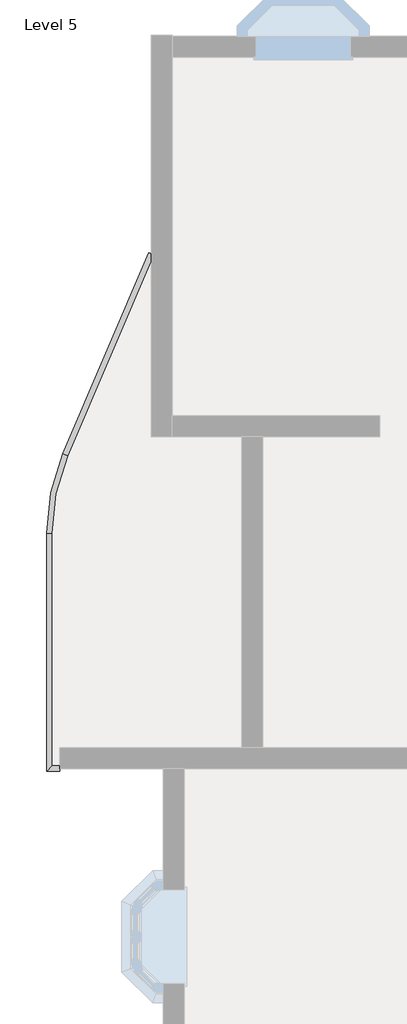
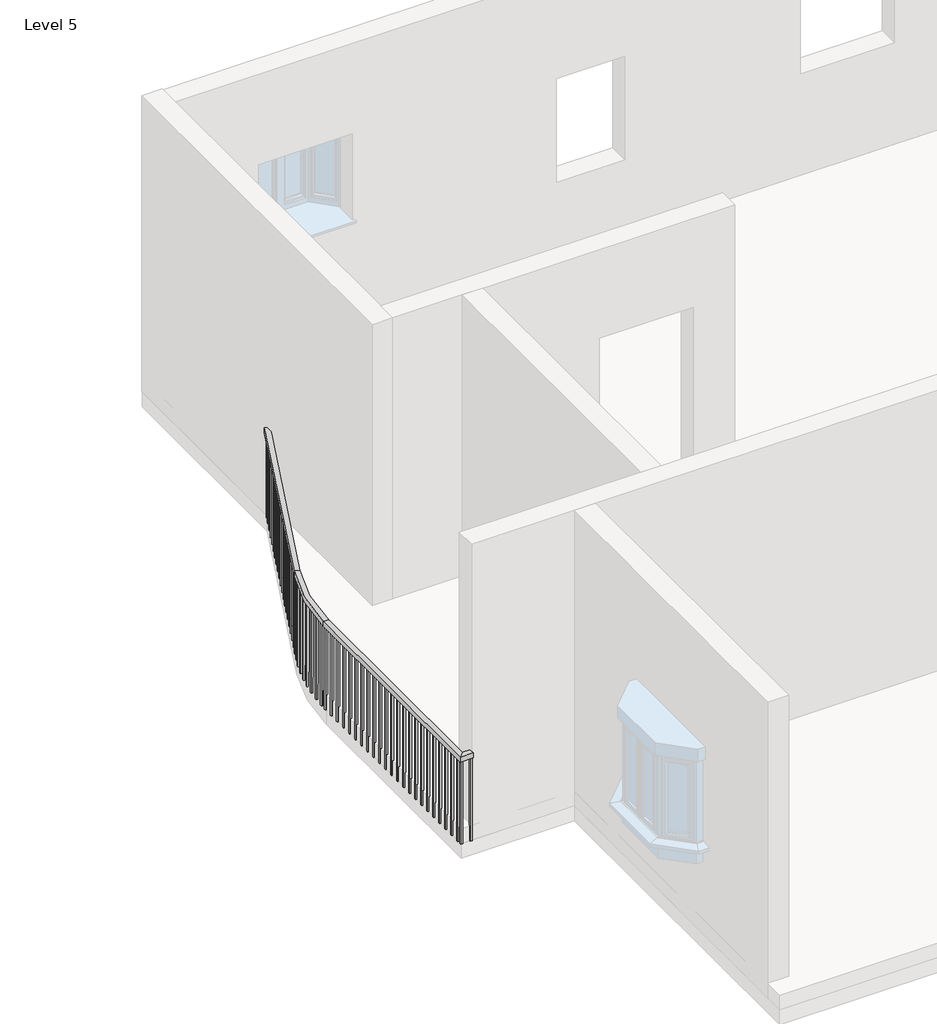
# One storey, part 7 of 14: 1 railing.
"""IFC4 building model written with IfcOpenShell, lengths in millimetres."""

from ifc_helpers import new_model, si_unit, frame, origin, place, context, project, spatial, polyline, circle_curve, outline, extrude, element, save
from ifc_brep_helpers import plane_surface, cylinder_surface, revolved_surface, advanced_brep

model = new_model("IFC4")

# Units and contexts
model_context = context("Model", 3, world=origin())
ifc_project = project(units=[si_unit("LENGTHUNIT", "METRE", prefix="MILLI")], contexts=[model_context])

# Site, building, storey
site = spatial("IfcSite", under=ifc_project)
building = spatial("IfcBuilding", under=site)
storey = spatial("IfcBuildingStorey", under=building, Name="Level 5", Elevation=12192.0)

# Railing
placement = place(None, origin())
element("IfcRailing", 1, ObjectType="Handrail - Rectangular", at=placement, inside=storey, context=model_context, shape_type="SolidModel", body=[
    advanced_brep(
    [(-12381.4379579, -2441.2590879, 13106.4), (-12381.4379579, -2441.2590879, 13055.6), (-12428.1364721, -2421.2618688, 13055.6), (-12428.1364721, -2421.2618688, 13106.4), (-13216.1814979, -4390.5942894, 13106.4), (-13216.1814979, -4390.5942894, 13055.6), (-13262.8800121, -4370.5970703, 13055.6), (-13262.8800121, -4370.5970703, 13106.4), (-13369.987215, -5140.4900045, 13055.6), (-13369.987215, -5140.4900045, 13106.4), (-13420.787215, -5140.4900045, 13055.6), (-13420.787215, -5140.4900045, 13106.4), (-13369.987215, -7396.5416506, 13106.4), (-13369.987215, -7396.5416506, 13055.6), (-13420.787215, -7447.3416506, 13055.6), (-13420.787215, -7447.3416506, 13106.4), (-13293.787215, -7396.5416506, 13106.4), (-13293.787215, -7447.3416506, 13106.4), (-13293.787215, -7447.3416506, 13055.6), (-13293.787215, -7396.5416506, 13055.6)],
    [
        (0, 1),
        (1, 2),
        (2, 3),
        (3, 0),
        (0, 4),
        (4, 5),
        (5, 1),
        (5, 6),
        (6, 2),
        (6, 7),
        (7, 3),
        (7, 4),
        (8, 5, circle_curve(frame((-11464.987215, -5140.4900045, 13055.6), z_axis=(0.0, 0.0, -1.0), x_axis=(-0.9192620907623801, 0.39364604467361003, 0.0)), 1905.0)),
        (4, 9, circle_curve(frame((-11464.987215, -5140.4900045, 13106.4), z_axis=(0.0, 0.0, 1.0), x_axis=(-0.9192620907623801, 0.39364604467361003, 0.0)), 1905.0)),
        (9, 8),
        (10, 6, circle_curve(frame((-11464.987215, -5140.4900045, 13055.6), z_axis=(0.0, 0.0, -1.0), x_axis=(-0.9192620907623801, 0.39364604467361003, 0.0)), 1955.8)),
        (8, 10),
        (11, 7, circle_curve(frame((-11464.987215, -5140.4900045, 13106.4), z_axis=(0.0, 0.0, -1.0), x_axis=(-0.9192620907623801, 0.39364604467361003, 0.0)), 1955.8)),
        (10, 11),
        (11, 9),
        (9, 12),
        (12, 13),
        (13, 8),
        (13, 14),
        (14, 10),
        (14, 15),
        (15, 11),
        (15, 12),
        (16, 17),
        (17, 18),
        (18, 19),
        (19, 16),
        (12, 16),
        (19, 13),
        (18, 14),
        (17, 15),
    ],
    [
        plane_surface(frame((-12404.787215, -2431.2604783, 13106.4), z_axis=(0.39364604467361003, 0.9192620907623801, 0.0), x_axis=(0.9192620907623801, -0.39364604467361003, 0.0))),
        plane_surface(frame((-12381.4379579, -2441.2590879, 13106.4), z_axis=(0.91926209076238, -0.39364604467361014, 0.0), x_axis=(-0.39364604467361014, -0.91926209076238, 0.0))),
        plane_surface(frame((-12381.4379579, -2441.2590879, 13055.6), z_axis=(0.0, 0.0, -1.0), x_axis=(-0.39364604467361014, -0.91926209076238, 0.0))),
        plane_surface(frame((-12428.1364721, -2421.2618688, 13055.6), z_axis=(-0.91926209076238, 0.39364604467361014, 0.0), x_axis=(-0.39364604467361014, -0.91926209076238, 0.0))),
        plane_surface(frame((-12428.1364721, -2421.2618688, 13106.4), z_axis=(0.0, 0.0, 1.0), x_axis=(-0.39364604467361014, -0.91926209076238, 0.0))),
        revolved_surface(polyline([(-13216.181497902333, -4390.594289396773, 13106.4), (-13216.181497902333, -4390.594289396773, 13055.6)]), (-11464.987215, -5140.4900045, 13106.4), (0.0, 0.0, 1.0)),
        plane_surface(frame((-11464.987215, -5140.4900045, 13055.6), z_axis=(0.0, 0.0, -1.0000000000000002), x_axis=(-0.9192620907623801, 0.39364604467361003, 0.0))),
        cylinder_surface(frame((-11464.987215, -5140.4900045, 13106.4), z_axis=(0.0, 0.0, 1.0), x_axis=(-0.9192620907623801, 0.39364604467361003, 0.0)), 1955.8),
        plane_surface(frame((-11464.987215, -5140.4900045, 13106.4), z_axis=(0.0, 0.0, 1.0000000000000002), x_axis=(-0.9192620907623801, 0.39364604467361003, 0.0))),
        plane_surface(frame((-13369.987215, -5140.4900045, 13106.4), z_axis=(1.0, 0.0, 0.0), x_axis=(0.0, -1.0, 0.0))),
        plane_surface(frame((-13369.987215, -5140.4900045, 13055.6), z_axis=(0.0, 0.0, -1.0), x_axis=(0.0, -1.0, 0.0))),
        plane_surface(frame((-13420.787215, -5140.4900045, 13055.6), z_axis=(-1.0, 0.0, 0.0), x_axis=(0.0, -1.0, 0.0))),
        plane_surface(frame((-13420.787215, -5140.4900045, 13106.4), z_axis=(0.0, 0.0, 1.0), x_axis=(0.0, -1.0, 0.0))),
        plane_surface(frame((-13293.787215, -7421.9416506, 13106.4), z_axis=(1.0, 0.0, 0.0), x_axis=(0.0, 1.0, 0.0))),
        plane_surface(frame((-13369.987215, -7396.5416506, 13106.4), z_axis=(0.0, 1.0, 0.0), x_axis=(1.0, 0.0, 0.0))),
        plane_surface(frame((-13369.987215, -7396.5416506, 13055.6), z_axis=(0.0, 0.0, -1.0), x_axis=(1.0, 0.0, 0.0))),
        plane_surface(frame((-13420.787215, -7447.3416506, 13055.6), z_axis=(0.0, -1.0, 0.0), x_axis=(1.0, 0.0, 0.0))),
        plane_surface(frame((-13420.787215, -7447.3416506, 13106.4), z_axis=(0.0, 0.0, 1.0), x_axis=(1.0, 0.0, 0.0))),
    ],
    [
        (0, [[1, 2, 3, 4]]),
        (1, [[-1, 5, 6, 7]]),
        (2, [[-2, -7, 8, 9]]),
        (3, [[-3, -9, 10, 11]]),
        (4, [[-4, -11, 12, -5]]),
        (5, [[13, -6, 14, 15]]),
        (6, [[16, -8, -13, 17]]),
        (7, [[18, -10, -16, 19]]),
        (8, [[-14, -12, -18, 20]]),
        (9, [[-15, 21, 22, 23]]),
        (10, [[-17, -23, 24, 25]]),
        (11, [[-19, -25, 26, 27]]),
        (12, [[-20, -27, 28, -21]]),
        (13, [[29, 30, 31, 32]]),
        (14, [[-22, 33, -32, 34]]),
        (15, [[-24, -34, -31, 35]]),
        (16, [[-26, -35, -30, 36]]),
        (17, [[-28, -36, -29, -33]]),
    ],
),
    extrude(outline(polyline([(-13404.912215, -7366.1650045), (-13385.862215, -7366.1650045), (-13385.862215, -7385.2150045), (-13404.912215, -7385.2150045), (-13404.912215, -7366.1650045)])), frame((0.0, 0.0, 12192.0), z_axis=(0.0, 0.0, 1.0), x_axis=(1.0, 0.0, 0.0)), (0.0, 0.0, 1.0), 863.6),
    extrude(outline(polyline([(-13404.912215, -7264.5650045), (-13385.862215, -7264.5650045), (-13385.862215, -7283.6150045), (-13404.912215, -7283.6150045), (-13404.912215, -7264.5650045)])), frame((0.0, 0.0, 12192.0), z_axis=(0.0, 0.0, 1.0), x_axis=(1.0, 0.0, 0.0)), (0.0, 0.0, 1.0), 863.6),
    extrude(outline(polyline([(-13404.912215, -7162.9650045), (-13385.862215, -7162.9650045), (-13385.862215, -7182.0150045), (-13404.912215, -7182.0150045), (-13404.912215, -7162.9650045)])), frame((0.0, 0.0, 12192.0), z_axis=(0.0, 0.0, 1.0), x_axis=(1.0, 0.0, 0.0)), (0.0, 0.0, 1.0), 863.6),
    extrude(outline(polyline([(-13404.912215, -7061.3650045), (-13385.862215, -7061.3650045), (-13385.862215, -7080.4150045), (-13404.912215, -7080.4150045), (-13404.912215, -7061.3650045)])), frame((0.0, 0.0, 12192.0), z_axis=(0.0, 0.0, 1.0), x_axis=(1.0, 0.0, 0.0)), (0.0, 0.0, 1.0), 863.6),
    extrude(outline(polyline([(-13404.912215, -6959.7650045), (-13385.862215, -6959.7650045), (-13385.862215, -6978.8150045), (-13404.912215, -6978.8150045), (-13404.912215, -6959.7650045)])), frame((0.0, 0.0, 12192.0), z_axis=(0.0, 0.0, 1.0), x_axis=(1.0, 0.0, 0.0)), (0.0, 0.0, 1.0), 863.6),
    extrude(outline(polyline([(-13404.912215, -6858.1650045), (-13385.862215, -6858.1650045), (-13385.862215, -6877.2150045), (-13404.912215, -6877.2150045), (-13404.912215, -6858.1650045)])), frame((0.0, 0.0, 12192.0), z_axis=(0.0, 0.0, 1.0), x_axis=(1.0, 0.0, 0.0)), (0.0, 0.0, 1.0), 863.6),
    extrude(outline(polyline([(-13404.912215, -6756.5650045), (-13385.862215, -6756.5650045), (-13385.862215, -6775.6150045), (-13404.912215, -6775.6150045), (-13404.912215, -6756.5650045)])), frame((0.0, 0.0, 12192.0), z_axis=(0.0, 0.0, 1.0), x_axis=(1.0, 0.0, 0.0)), (0.0, 0.0, 1.0), 863.6),
    extrude(outline(polyline([(-13404.912215, -6654.9650045), (-13385.862215, -6654.9650045), (-13385.862215, -6674.0150045), (-13404.912215, -6674.0150045), (-13404.912215, -6654.9650045)])), frame((0.0, 0.0, 12192.0), z_axis=(0.0, 0.0, 1.0), x_axis=(1.0, 0.0, 0.0)), (0.0, 0.0, 1.0), 863.6),
    extrude(outline(polyline([(-13404.912215, -6553.3650045), (-13385.862215, -6553.3650045), (-13385.862215, -6572.4150045), (-13404.912215, -6572.4150045), (-13404.912215, -6553.3650045)])), frame((0.0, 0.0, 12192.0), z_axis=(0.0, 0.0, 1.0), x_axis=(1.0, 0.0, 0.0)), (0.0, 0.0, 1.0), 863.6),
    extrude(outline(polyline([(-13404.912215, -6451.7650045), (-13385.862215, -6451.7650045), (-13385.862215, -6470.8150045), (-13404.912215, -6470.8150045), (-13404.912215, -6451.7650045)])), frame((0.0, 0.0, 12192.0), z_axis=(0.0, 0.0, 1.0), x_axis=(1.0, 0.0, 0.0)), (0.0, 0.0, 1.0), 863.6),
    extrude(outline(polyline([(-13404.912215, -6350.1650045), (-13385.862215, -6350.1650045), (-13385.862215, -6369.2150045), (-13404.912215, -6369.2150045), (-13404.912215, -6350.1650045)])), frame((0.0, 0.0, 12192.0), z_axis=(0.0, 0.0, 1.0), x_axis=(1.0, 0.0, 0.0)), (0.0, 0.0, 1.0), 863.6),
    extrude(outline(polyline([(-13404.912215, -6248.5650045), (-13385.862215, -6248.5650045), (-13385.862215, -6267.6150045), (-13404.912215, -6267.6150045), (-13404.912215, -6248.5650045)])), frame((0.0, 0.0, 12192.0), z_axis=(0.0, 0.0, 1.0), x_axis=(1.0, 0.0, 0.0)), (0.0, 0.0, 1.0), 863.6),
    extrude(outline(polyline([(-13404.912215, -6146.9650045), (-13385.862215, -6146.9650045), (-13385.862215, -6166.0150045), (-13404.912215, -6166.0150045), (-13404.912215, -6146.9650045)])), frame((0.0, 0.0, 12192.0), z_axis=(0.0, 0.0, 1.0), x_axis=(1.0, 0.0, 0.0)), (0.0, 0.0, 1.0), 863.6),
    extrude(outline(polyline([(-13404.912215, -6045.3650045), (-13385.862215, -6045.3650045), (-13385.862215, -6064.4150045), (-13404.912215, -6064.4150045), (-13404.912215, -6045.3650045)])), frame((0.0, 0.0, 12192.0), z_axis=(0.0, 0.0, 1.0), x_axis=(1.0, 0.0, 0.0)), (0.0, 0.0, 1.0), 863.6),
    extrude(outline(polyline([(-13404.912215, -5943.7650045), (-13385.862215, -5943.7650045), (-13385.862215, -5962.8150045), (-13404.912215, -5962.8150045), (-13404.912215, -5943.7650045)])), frame((0.0, 0.0, 12192.0), z_axis=(0.0, 0.0, 1.0), x_axis=(1.0, 0.0, 0.0)), (0.0, 0.0, 1.0), 863.6),
    extrude(outline(polyline([(-13404.912215, -5842.1650045), (-13385.862215, -5842.1650045), (-13385.862215, -5861.2150045), (-13404.912215, -5861.2150045), (-13404.912215, -5842.1650045)])), frame((0.0, 0.0, 12192.0), z_axis=(0.0, 0.0, 1.0), x_axis=(1.0, 0.0, 0.0)), (0.0, 0.0, 1.0), 863.6),
    extrude(outline(polyline([(-13404.912215, -5740.5650045), (-13385.862215, -5740.5650045), (-13385.862215, -5759.6150045), (-13404.912215, -5759.6150045), (-13404.912215, -5740.5650045)])), frame((0.0, 0.0, 12192.0), z_axis=(0.0, 0.0, 1.0), x_axis=(1.0, 0.0, 0.0)), (0.0, 0.0, 1.0), 863.6),
    extrude(outline(polyline([(-13404.912215, -5638.9650045), (-13385.862215, -5638.9650045), (-13385.862215, -5658.0150045), (-13404.912215, -5658.0150045), (-13404.912215, -5638.9650045)])), frame((0.0, 0.0, 12192.0), z_axis=(0.0, 0.0, 1.0), x_axis=(1.0, 0.0, 0.0)), (0.0, 0.0, 1.0), 863.6),
    extrude(outline(polyline([(-13404.912215, -5537.3650045), (-13385.862215, -5537.3650045), (-13385.862215, -5556.4150045), (-13404.912215, -5556.4150045), (-13404.912215, -5537.3650045)])), frame((0.0, 0.0, 12192.0), z_axis=(0.0, 0.0, 1.0), x_axis=(1.0, 0.0, 0.0)), (0.0, 0.0, 1.0), 863.6),
    extrude(outline(polyline([(-13404.912215, -5435.7650045), (-13385.862215, -5435.7650045), (-13385.862215, -5454.8150045), (-13404.912215, -5454.8150045), (-13404.912215, -5435.7650045)])), frame((0.0, 0.0, 12192.0), z_axis=(0.0, 0.0, 1.0), x_axis=(1.0, 0.0, 0.0)), (0.0, 0.0, 1.0), 863.6),
    extrude(outline(polyline([(-13404.912215, -5334.1650045), (-13385.862215, -5334.1650045), (-13385.862215, -5353.2150045), (-13404.912215, -5353.2150045), (-13404.912215, -5334.1650045)])), frame((0.0, 0.0, 12192.0), z_axis=(0.0, 0.0, 1.0), x_axis=(1.0, 0.0, 0.0)), (0.0, 0.0, 1.0), 863.6),
    extrude(outline(polyline([(-13404.912215, -5232.5650045), (-13385.862215, -5232.5650045), (-13385.862215, -5251.6150045), (-13404.912215, -5251.6150045), (-13404.912215, -5232.5650045)])), frame((0.0, 0.0, 12192.0), z_axis=(0.0, 0.0, 1.0), x_axis=(1.0, 0.0, 0.0)), (0.0, 0.0, 1.0), 863.6),
    extrude(outline(polyline([(-13403.2986616, -5060.8127369), (-13384.2611239, -5061.5016911), (-13384.9500781, -5080.5392288), (-13403.9876158, -5079.8502746), (-13403.2986616, -5060.8127369)])), frame((0.0, 0.0, 12192.0), z_axis=(0.0, 0.0, 1.0), x_axis=(1.0, 0.0, 0.0)), (0.0, 0.0, 1.0), 863.6),
    extrude(outline(polyline([(-13396.4230348, -4958.9537683), (-13377.4481028, -4960.6432816), (-13379.1376161, -4979.6182136), (-13398.1125481, -4977.9287003), (-13396.4230348, -4958.9537683)])), frame((0.0, 0.0, 12192.0), z_axis=(0.0, 0.0, 1.0), x_axis=(1.0, 0.0, 0.0)), (0.0, 0.0, 1.0), 863.6),
    extrude(outline(polyline([(-13384.1984052, -4857.5975541), (-13365.3386289, -4860.2829475), (-13368.0240223, -4879.1427238), (-13386.8837986, -4876.4573304), (-13384.1984052, -4857.5975541)])), frame((0.0, 0.0, 12192.0), z_axis=(0.0, 0.0, 1.0), x_axis=(1.0, 0.0, 0.0)), (0.0, 0.0, 1.0), 863.6),
    extrude(outline(polyline([(-13366.6586282, -4757.0247946), (-13347.9662387, -4760.698631), (-13351.6400752, -4779.3910205), (-13370.3324647, -4775.7171841), (-13366.6586282, -4757.0247946)])), frame((0.0, 0.0, 12192.0), z_axis=(0.0, 0.0, 1.0), x_axis=(1.0, 0.0, 0.0)), (0.0, 0.0, 1.0), 863.6),
    extrude(outline(polyline([(-13343.8522793, -4657.5140204), (-13325.3790441, -4662.1661254), (-13330.0311492, -4680.6393606), (-13348.5043844, -4675.9872556), (-13343.8522793, -4657.5140204)])), frame((0.0, 0.0, 12192.0), z_axis=(0.0, 0.0, 1.0), x_axis=(1.0, 0.0, 0.0)), (0.0, 0.0, 1.0), 863.6),
    extrude(outline(polyline([(-13315.8425193, -4559.340821), (-13297.6395991, -4564.9583109), (-13303.257089, -4583.1612312), (-13321.4600093, -4577.5437413), (-13315.8425193, -4559.340821)])), frame((0.0, 0.0, 12192.0), z_axis=(0.0, 0.0, 1.0), x_axis=(1.0, 0.0, 0.0)), (0.0, 0.0, 1.0), 863.6),
    extrude(outline(polyline([(-13282.7069198, -4462.7770815), (-13264.8247264, -4469.344399), (-13271.3920438, -4487.2265924), (-13289.2742372, -4480.659275), (-13282.7069198, -4462.7770815)])), frame((0.0, 0.0, 12192.0), z_axis=(0.0, 0.0, 1.0), x_axis=(1.0, 0.0, 0.0)), (0.0, 0.0, 1.0), 863.6),
    extrude(outline(polyline([(-13209.6824706, -4286.6955968), (-13192.1705278, -4294.1945539), (-13199.6694849, -4311.7064967), (-13217.1814277, -4304.2075396), (-13209.6824706, -4286.6955968)])), frame((0.0, 0.0, 12192.0), z_axis=(0.0, 0.0, 1.0), x_axis=(1.0, 0.0, 0.0)), (0.0, 0.0, 1.0), 863.6),
    extrude(outline(polyline([(-13169.6880325, -4193.2985683), (-13152.1760896, -4200.7975255), (-13159.6750468, -4218.3094683), (-13177.1869896, -4210.8105112), (-13169.6880325, -4193.2985683)])), frame((0.0, 0.0, 12192.0), z_axis=(0.0, 0.0, 1.0), x_axis=(1.0, 0.0, 0.0)), (0.0, 0.0, 1.0), 863.6),
    extrude(outline(polyline([(-13129.6935943, -4099.9015399), (-13112.1816515, -4107.4004971), (-13119.6806086, -4124.9124399), (-13137.1925515, -4117.4134827), (-13129.6935943, -4099.9015399)])), frame((0.0, 0.0, 12192.0), z_axis=(0.0, 0.0, 1.0), x_axis=(1.0, 0.0, 0.0)), (0.0, 0.0, 1.0), 863.6),
    extrude(outline(polyline([(-13089.6991562, -4006.5045115), (-13072.1872133, -4014.0034686), (-13079.6861705, -4031.5154115), (-13097.1981133, -4024.0164543), (-13089.6991562, -4006.5045115)])), frame((0.0, 0.0, 12192.0), z_axis=(0.0, 0.0, 1.0), x_axis=(1.0, 0.0, 0.0)), (0.0, 0.0, 1.0), 863.6),
    extrude(outline(polyline([(-13049.704718, -3913.1074831), (-13032.1927752, -3920.6064402), (-13039.6917324, -3938.1183831), (-13057.2036752, -3930.6194259), (-13049.704718, -3913.1074831)])), frame((0.0, 0.0, 12192.0), z_axis=(0.0, 0.0, 1.0), x_axis=(1.0, 0.0, 0.0)), (0.0, 0.0, 1.0), 863.6),
    extrude(outline(polyline([(-13009.7102799, -3819.7104546), (-12992.1983371, -3827.2094118), (-12999.6972942, -3844.7213546), (-13017.209237, -3837.2223975), (-13009.7102799, -3819.7104546)])), frame((0.0, 0.0, 12192.0), z_axis=(0.0, 0.0, 1.0), x_axis=(1.0, 0.0, 0.0)), (0.0, 0.0, 1.0), 863.6),
    extrude(outline(polyline([(-12969.7158418, -3726.3134262), (-12952.2038989, -3733.8123834), (-12959.7028561, -3751.3243262), (-12977.2147989, -3743.8253691), (-12969.7158418, -3726.3134262)])), frame((0.0, 0.0, 12192.0), z_axis=(0.0, 0.0, 1.0), x_axis=(1.0, 0.0, 0.0)), (0.0, 0.0, 1.0), 863.6),
    extrude(outline(polyline([(-12929.7214036, -3632.9163978), (-12912.2094608, -3640.415355), (-12919.7084179, -3657.9272978), (-12937.2203608, -3650.4283406), (-12929.7214036, -3632.9163978)])), frame((0.0, 0.0, 12192.0), z_axis=(0.0, 0.0, 1.0), x_axis=(1.0, 0.0, 0.0)), (0.0, 0.0, 1.0), 863.6),
    extrude(outline(polyline([(-12889.7269655, -3539.5193694), (-12872.2150227, -3547.0183265), (-12879.7139798, -3564.5302694), (-12897.2259226, -3557.0313122), (-12889.7269655, -3539.5193694)])), frame((0.0, 0.0, 12192.0), z_axis=(0.0, 0.0, 1.0), x_axis=(1.0, 0.0, 0.0)), (0.0, 0.0, 1.0), 863.6),
    extrude(outline(polyline([(-12849.7325273, -3446.122341), (-12832.2205845, -3453.6212981), (-12839.7195417, -3471.1332409), (-12857.2314845, -3463.6342838), (-12849.7325273, -3446.122341)])), frame((0.0, 0.0, 12192.0), z_axis=(0.0, 0.0, 1.0), x_axis=(1.0, 0.0, 0.0)), (0.0, 0.0, 1.0), 863.6),
    extrude(outline(polyline([(-12809.7380892, -3352.7253125), (-12792.2261464, -3360.2242697), (-12799.7251035, -3377.7362125), (-12817.2370464, -3370.2372554), (-12809.7380892, -3352.7253125)])), frame((0.0, 0.0, 12192.0), z_axis=(0.0, 0.0, 1.0), x_axis=(1.0, 0.0, 0.0)), (0.0, 0.0, 1.0), 863.6),
    extrude(outline(polyline([(-12769.7436511, -3259.3282841), (-12752.2317082, -3266.8272413), (-12759.7306654, -3284.3391841), (-12777.2426082, -3276.8402269), (-12769.7436511, -3259.3282841)])), frame((0.0, 0.0, 12192.0), z_axis=(0.0, 0.0, 1.0), x_axis=(1.0, 0.0, 0.0)), (0.0, 0.0, 1.0), 863.6),
    extrude(outline(polyline([(-12729.7492129, -3165.9312557), (-12712.2372701, -3173.4302129), (-12719.7362272, -3190.9421557), (-12737.2481701, -3183.4431985), (-12729.7492129, -3165.9312557)])), frame((0.0, 0.0, 12192.0), z_axis=(0.0, 0.0, 1.0), x_axis=(1.0, 0.0, 0.0)), (0.0, 0.0, 1.0), 863.6),
    extrude(outline(polyline([(-12689.7547748, -3072.5342273), (-12672.242832, -3080.0331844), (-12679.7417891, -3097.5451273), (-12697.2537319, -3090.0461701), (-12689.7547748, -3072.5342273)])), frame((0.0, 0.0, 12192.0), z_axis=(0.0, 0.0, 1.0), x_axis=(1.0, 0.0, 0.0)), (0.0, 0.0, 1.0), 863.6),
    extrude(outline(polyline([(-12649.7603366, -2979.1371989), (-12632.2483938, -2986.636156), (-12639.747351, -3004.1480988), (-12657.2592938, -2996.6491417), (-12649.7603366, -2979.1371989)])), frame((0.0, 0.0, 12192.0), z_axis=(0.0, 0.0, 1.0), x_axis=(1.0, 0.0, 0.0)), (0.0, 0.0, 1.0), 863.6),
    extrude(outline(polyline([(-12609.7658985, -2885.7401704), (-12592.2539557, -2893.2391276), (-12599.7529128, -2910.7510704), (-12617.2648557, -2903.2521133), (-12609.7658985, -2885.7401704)])), frame((0.0, 0.0, 12192.0), z_axis=(0.0, 0.0, 1.0), x_axis=(1.0, 0.0, 0.0)), (0.0, 0.0, 1.0), 863.6),
    extrude(outline(polyline([(-12569.7714604, -2792.343142), (-12552.2595175, -2799.8420992), (-12559.7584747, -2817.354042), (-12577.2704175, -2809.8550848), (-12569.7714604, -2792.343142)])), frame((0.0, 0.0, 12192.0), z_axis=(0.0, 0.0, 1.0), x_axis=(1.0, 0.0, 0.0)), (0.0, 0.0, 1.0), 863.6),
    extrude(outline(polyline([(-12529.7770222, -2698.9461136), (-12512.2650794, -2706.4450707), (-12519.7640366, -2723.9570136), (-12537.2759794, -2716.4580564), (-12529.7770222, -2698.9461136)])), frame((0.0, 0.0, 12192.0), z_axis=(0.0, 0.0, 1.0), x_axis=(1.0, 0.0, 0.0)), (0.0, 0.0, 1.0), 863.6),
    extrude(outline(polyline([(-12489.7825841, -2605.5490852), (-12472.2706413, -2613.0480423), (-12479.7695984, -2630.5599852), (-12497.2815412, -2623.061028), (-12489.7825841, -2605.5490852)])), frame((0.0, 0.0, 12192.0), z_axis=(0.0, 0.0, 1.0), x_axis=(1.0, 0.0, 0.0)), (0.0, 0.0, 1.0), 863.6),
    extrude(outline(polyline([(-12449.788146, -2512.1520567), (-12432.2762031, -2519.6510139), (-12439.7751603, -2537.1629567), (-12457.2871031, -2529.6639996), (-12449.788146, -2512.1520567)])), frame((0.0, 0.0, 12192.0), z_axis=(0.0, 0.0, 1.0), x_axis=(1.0, 0.0, 0.0)), (0.0, 0.0, 1.0), 863.6),
    extrude(outline(polyline([(-13404.912215, -7412.4166506), (-13385.862215, -7412.4166506), (-13385.862215, -7431.4666506), (-13404.912215, -7431.4666506), (-13404.912215, -7412.4166506)])), frame((0.0, 0.0, 12192.0), z_axis=(0.0, 0.0, 1.0), x_axis=(1.0, 0.0, 0.0)), (0.0, 0.0, 1.0), 863.6),
    extrude(outline(polyline([(-13404.912215, -5130.9650045), (-13385.862215, -5130.9650045), (-13385.862215, -5150.0150045), (-13404.912215, -5150.0150045), (-13404.912215, -5130.9650045)])), frame((0.0, 0.0, 12192.0), z_axis=(0.0, 0.0, 1.0), x_axis=(1.0, 0.0, 0.0)), (0.0, 0.0, 1.0), 863.6),
    extrude(outline(polyline([(-13244.5372478, -4368.0902299), (-13227.025305, -4375.589187), (-13234.5242621, -4393.1011299), (-13252.036205, -4385.6021727), (-13244.5372478, -4368.0902299)])), frame((0.0, 0.0, 12192.0), z_axis=(0.0, 0.0, 1.0), x_axis=(1.0, 0.0, 0.0)), (0.0, 0.0, 1.0), 863.6),
    extrude(outline(polyline([(-13312.837215, -7431.4666506), (-13312.837215, -7412.4166506), (-13293.787215, -7412.4166506), (-13293.787215, -7431.4666506), (-13312.837215, -7431.4666506)])), frame((0.0, 0.0, 12192.0), z_axis=(0.0, 0.0, 1.0), x_axis=(1.0, 0.0, 0.0)), (0.0, 0.0, 1.0), 863.6),
    extrude(outline(polyline([(-12413.5431864, -2427.5109997), (-12396.0312436, -2435.0099569), (-12403.5302007, -2452.5218997), (-12421.0421435, -2445.0229426), (-12413.5431864, -2427.5109997)])), frame((0.0, 0.0, 12192.0), z_axis=(0.0, 0.0, 1.0), x_axis=(1.0, 0.0, 0.0)), (0.0, 0.0, 1.0), 863.6),
])

save(model, "model.ifc")

# Revit data of these elements
# Type "Handrail - Rectangular"
#   Assembly Code = "C2010400"
#   built-in parameter 1008612 = 0.0416667 (stored number, unit not read)
#   built-in parameter 1008611 = 0.0416667 (stored number, unit not read)
#   built-in parameter 1008609 = 0.333333 (stored number, unit not read)
#   built-in parameter 1008604 = 0.166667 (stored number, unit not read)
#   built-in parameter 1008603 = 0.166667 (stored number, unit not read)
#   Railing Height = 3' - 0"
#   built-in parameter 1008630 = 2
#   built-in parameter 1008610 = 2
#   built-in parameter 1008618 = Baluster - Square : 3/4"
# Element 1 (IfcRailing, "Handrail - Rectangular")
#   Phase Created = New Construction
